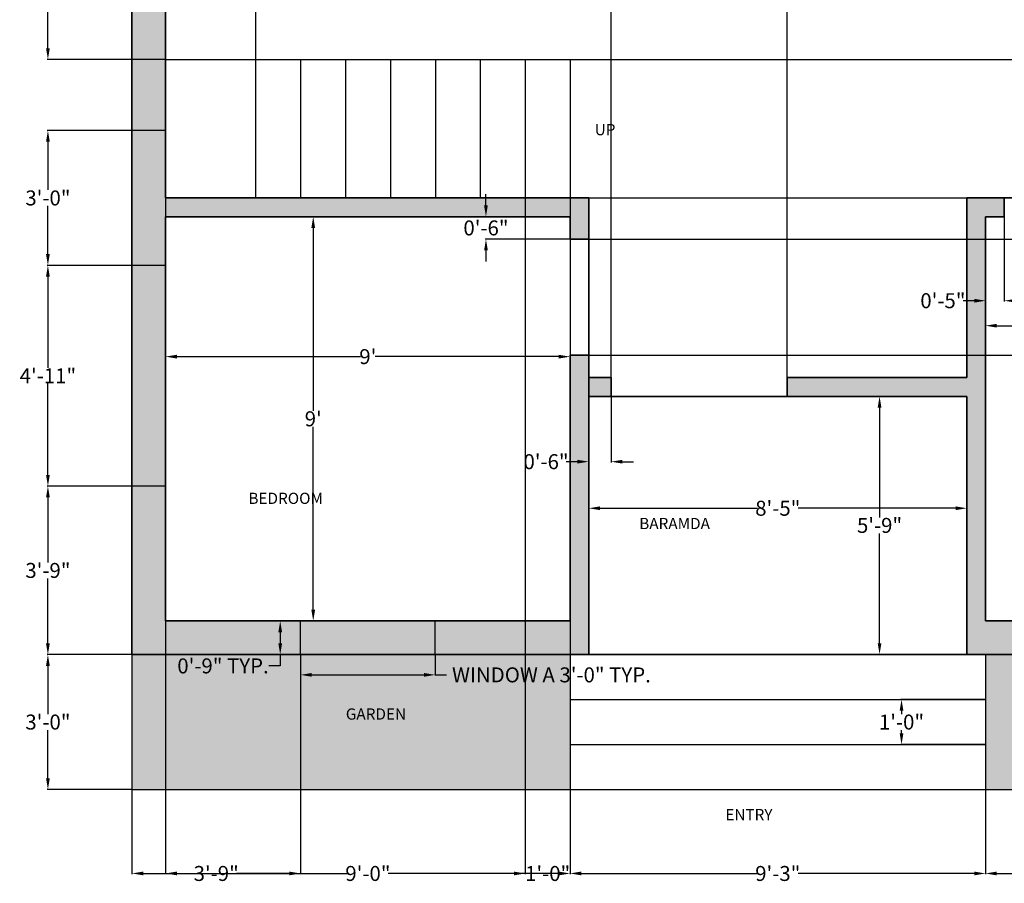
# Model space of a CAD drawing. Units: inches. Extents: x 477 to 929, y 265 to 727.
# Tile 1 of 4: x 477 to 740, y 265 to 496. Entities that reach past the tile are written whole.
import ezdxf

# ---------------------------------------------------------------- set-up
doc = ezdxf.new("R2010")
doc.units = ezdxf.units.IN
doc.header["$MEASUREMENT"] = 0
for name, color, linetype, lineweight, true_color in [('A-ANNO-DIMS', 215, 'Continuous', 18, 0xa953a0), ('A-WALL-PATT', 244, 'Continuous', 13, 0x991b1e), ('L-PLNT-PATT', 114, 'Continuous', 13, 0x139b48)]:
    doc.layers.add(name, color=color, linetype=linetype, lineweight=lineweight, true_color=true_color)
for name, color, linetype, lineweight in [('A-ANNO-TEXT', 3, 'Continuous', 18), ('A-AREA-IDEN', 3, 'Continuous', 25), ('A-FLOR-STRS', 7, 'Continuous', 25), ('A-GLAZ', 4, 'Continuous', 25), ('A-GLAZ-PATT', 7, 'Continuous', 13), ('A-WALL', 7, 'Continuous', 35), ('L-SITE', 7, 'Continuous', 25)]:
    doc.layers.add(name, color=color, linetype=linetype, lineweight=lineweight)
doc.styles.get("Standard").update_dxf_attribs({"font": 'arial.ttf'})
doc.dimstyles.get("Standard").update_dxf_attribs({"dimtxt": 4, "dimasz": 3, "dimexe": 0.18, "dimexo": 0.0625, "dimgap": 0.09, "dimtad": 0, "dimtih": 1, "dimtoh": 1, "dimdec": 0, "dimzin": 0, "dimdsep": 46, "dimlunit": 3, "dimtxsty": 'Standard', "dimcen": 0, "dimadec": 0, "dimazin": 0, "dimtfac": 1, "dimtdec": 0, "dimtofl": 0, "dimtmove": 0, "dimatfit": 3, "dimfxl": 1, "dimtolj": 1, "dimtzin": 0, "dimarcsym": 1})

# ---------------------------------------------------------------- blocks, each defined once
blk = doc.blocks.new('*D1')
at = {"layer": 'A-ANNO-DIMS', "color": 0, "lineweight": -2, "transparency": 16777216}
for p, q in [((553.16, 443.21), (555.92, 443.21)), ((555.74, 440.21), (555.74, 391.34)), ((555.74, 338.21), (555.74, 387.07)), ((555.8, 335.21), (555.92, 335.21))]:
    blk.add_line(p, q, dxfattribs=at)
at = {"layer": 'A-ANNO-DIMS', "color": 0, "transparency": 16777216}
for points in [[(555.24, 440.21), (556.24, 440.21), (555.74, 443.21)], [(555.24, 338.21), (556.24, 338.21), (555.74, 335.21)]]:
    blk.add_solid(points, dxfattribs=at)
at = {"layer": 'Defpoints', "color": 0, "transparency": 16777216}
for p in [(553.09, 443.21), (555.74, 335.21), (555.74, 335.21)]:
    blk.add_point(p, dxfattribs=at)
at = {"layer": 'A-ANNO-DIMS', "color": 0, "transparency": 16777216, "insert": (555.74, 389.21), "char_height": 4, "attachment_point": 5}
blk.add_mtext("\\A1;9'", dxfattribs=at)
blk = doc.blocks.new('*D2')
at = {"layer": 'A-ANNO-DIMS', "color": 0, "lineweight": -2, "transparency": 16777216}
for p, q in [((516.33, 389.27), (516.33, 406)), ((519.33, 405.82), (568.4, 405.82)), ((621.33, 405.82), (572.26, 405.82)), ((624.33, 389.27), (624.33, 406))]:
    blk.add_line(p, q, dxfattribs=at)
at = {"layer": 'A-ANNO-DIMS', "color": 0, "transparency": 16777216}
for points in [[(519.33, 406.32), (519.33, 405.32), (516.33, 405.82)], [(621.33, 406.32), (621.33, 405.32), (624.33, 405.82)]]:
    blk.add_solid(points, dxfattribs=at)
at = {"layer": 'Defpoints', "color": 0, "transparency": 16777216}
for p in [(624.33, 405.82), (516.33, 389.21), (624.33, 389.21)]:
    blk.add_point(p, dxfattribs=at)
at = {"layer": 'A-ANNO-DIMS', "color": 0, "transparency": 16777216, "insert": (570.33, 405.82), "char_height": 4, "attachment_point": 5}
blk.add_mtext("\\A1;9'", dxfattribs=at)
blk = doc.blocks.new('*D3')
at = {"layer": 'A-ANNO-DIMS', "color": 0, "lineweight": -2, "transparency": 16777216}
for p, q in [((629.33, 326.27), (629.33, 365.5)), ((632.33, 365.32), (674.42, 365.32)), ((727.33, 365.32), (685.24, 365.32)), ((730.33, 326.27), (730.33, 365.5))]:
    blk.add_line(p, q, dxfattribs=at)
at = {"layer": 'A-ANNO-DIMS', "color": 0, "transparency": 16777216}
for points in [[(632.33, 365.82), (632.33, 364.82), (629.33, 365.32)], [(727.33, 365.82), (727.33, 364.82), (730.33, 365.32)]]:
    blk.add_solid(points, dxfattribs=at)
at = {"layer": 'Defpoints', "color": 0, "transparency": 16777216}
for p in [(730.33, 365.32), (629.33, 326.21), (730.33, 326.21)]:
    blk.add_point(p, dxfattribs=at)
at = {"layer": 'A-ANNO-DIMS', "color": 0, "transparency": 16777216, "insert": (679.83, 365.32), "char_height": 4, "attachment_point": 5}
blk.add_mtext('\\A1;8\'-5"', dxfattribs=at)
blk = doc.blocks.new('*D4')
at = {"layer": 'A-ANNO-DIMS', "color": 0, "lineweight": -2, "transparency": 16777216}
for p, q in [((730.27, 395.21), (706.83, 395.21)), ((707.01, 392.21), (707.01, 362.87)), ((707.01, 329.27), (707.01, 358.6)), ((730.27, 326.27), (706.83, 326.27))]:
    blk.add_line(p, q, dxfattribs=at)
at = {"layer": 'A-ANNO-DIMS', "color": 0, "transparency": 16777216}
for points in [[(706.51, 392.21), (707.51, 392.21), (707.01, 395.21)], [(706.51, 329.27), (707.51, 329.27), (707.01, 326.27)]]:
    blk.add_solid(points, dxfattribs=at)
at = {"layer": 'Defpoints', "color": 0, "transparency": 16777216}
for p in [(730.33, 395.21), (707.01, 326.27), (730.33, 326.27)]:
    blk.add_point(p, dxfattribs=at)
at = {"layer": 'A-ANNO-DIMS', "color": 0, "transparency": 16777216, "insert": (707.01, 360.74), "char_height": 4, "attachment_point": 5}
blk.add_mtext('\\A1;5\'-9"', dxfattribs=at)
blk = doc.blocks.new('*D5')
at = {"layer": 'A-ANNO-DIMS', "color": 0, "lineweight": -2, "transparency": 16777216}
for p, q in [((735.33, 335.27), (735.33, 414.27)), ((738.33, 414.09), (796.06, 414.09)), ((867.33, 414.09), (809.61, 414.09)), ((870.33, 335.27), (870.33, 414.27))]:
    blk.add_line(p, q, dxfattribs=at)
at = {"layer": 'A-ANNO-DIMS', "color": 0, "transparency": 16777216}
for points in [[(738.33, 414.59), (738.33, 413.59), (735.33, 414.09)], [(867.33, 414.59), (867.33, 413.59), (870.33, 414.09)]]:
    blk.add_solid(points, dxfattribs=at)
at = {"layer": 'Defpoints', "color": 0, "transparency": 16777216}
for p in [(870.33, 414.09), (735.33, 335.21), (870.33, 335.21)]:
    blk.add_point(p, dxfattribs=at)
at = {"layer": 'A-ANNO-DIMS', "color": 0, "transparency": 16777216, "insert": (802.83, 414.09), "char_height": 4, "attachment_point": 5}
blk.add_mtext('\\A1;11\'-3"', dxfattribs=at)
blk = doc.blocks.new('WIN-JAMBS-36IN')
for p, q in [((9, 36), (0, 36)), ((9, 0), (0, 0))]:
    blk.add_line(p, q)
blk = doc.blocks.new('*D23')
at = {"layer": 'A-ANNO-DIMS', "color": 0, "lineweight": -2, "transparency": 16777216}
for p, q in [((552.33, 326.14), (552.33, 320.63)), ((588.33, 326.14), (588.33, 320.63)), ((555.33, 320.81), (585.33, 320.81)), ((588.33, 320.81), (591.33, 320.81))]:
    blk.add_line(p, q, dxfattribs=at)
at = {"layer": 'A-ANNO-DIMS', "color": 0, "transparency": 16777216}
for points in [[(555.33, 321.31), (555.33, 320.31), (552.33, 320.81)], [(585.33, 321.31), (585.33, 320.31), (588.33, 320.81)]]:
    blk.add_solid(points, dxfattribs=at)
at = {"layer": 'Defpoints', "color": 0, "transparency": 16777216}
for p in [(552.33, 326.21), (588.33, 326.21), (588.33, 320.81)]:
    blk.add_point(p, dxfattribs=at)
at = {"layer": 'A-ANNO-DIMS', "color": 0, "transparency": 16777216, "insert": (619.37, 320.81), "char_height": 4, "attachment_point": 5}
blk.add_mtext('\\A1;WINDOW A 3\'-0" TYP.', dxfattribs=at)
blk = doc.blocks.new('*D24')
at = {"layer": 'A-ANNO-DIMS', "color": 0, "lineweight": -2, "transparency": 16777216}
for p, q in [((552.27, 335.21), (546.75, 335.21)), ((546.93, 332.21), (546.93, 329.21)), ((552.27, 326.21), (546.75, 326.21)), ((546.93, 326.21), (546.93, 323.21)), ((546.93, 323.21), (543.93, 323.21))]:
    blk.add_line(p, q, dxfattribs=at)
at = {"layer": 'A-ANNO-DIMS', "color": 0, "transparency": 16777216}
for points in [[(546.43, 332.21), (547.43, 332.21), (546.93, 335.21)], [(546.43, 329.21), (547.43, 329.21), (546.93, 326.21)]]:
    blk.add_solid(points, dxfattribs=at)
at = {"layer": 'Defpoints', "color": 0, "transparency": 16777216}
for p in [(552.33, 335.21), (546.93, 326.21), (552.33, 326.21)]:
    blk.add_point(p, dxfattribs=at)
at = {"layer": 'A-ANNO-DIMS', "color": 0, "transparency": 16777216, "insert": (531.65, 323.21), "char_height": 4, "attachment_point": 5}
blk.add_mtext('\\A1;0\'-9" TYP.', dxfattribs=at)
blk = doc.blocks.new('*D29')
at = {"layer": 'A-ANNO-DIMS', "color": 0, "lineweight": -2, "transparency": 16777216}
for p, q in [((624.43, 485.21), (901.96, 485.21)), ((901.78, 482.21), (901.78, 468.84)), ((901.78, 451.21), (901.78, 464.57)), ((624.43, 448.21), (901.96, 448.21))]:
    blk.add_line(p, q, dxfattribs=at)
at = {"layer": 'A-ANNO-DIMS', "color": 0, "transparency": 16777216}
for points in [[(901.28, 482.21), (902.28, 482.21), (901.78, 485.21)], [(901.28, 451.21), (902.28, 451.21), (901.78, 448.21)]]:
    blk.add_solid(points, dxfattribs=at)
at = {"layer": 'Defpoints', "color": 0, "transparency": 16777216}
for p in [(624.37, 485.21), (901.78, 485.21), (624.37, 448.21)]:
    blk.add_point(p, dxfattribs=at)
at = {"layer": 'A-ANNO-DIMS', "color": 0, "transparency": 16777216, "insert": (901.78, 466.71), "char_height": 4, "attachment_point": 5}
blk.add_mtext('\\A1;3\'-1"', dxfattribs=at)
blk = doc.blocks.new('*D31')
at = {"layer": 'A-ANNO-DIMS', "color": 0, "lineweight": -2, "transparency": 16777216}
for p, q in [((612.368072, 485.142663), (612.368072, 267.575163)), ((624.368072, 485.142663), (624.368072, 267.575163)), ((609.368072, 267.755163), (606.368072, 267.755163)), ((627.368072, 267.755163), (630.368072, 267.755163))]:
    blk.add_line(p, q, dxfattribs=at)
at = {"layer": 'A-ANNO-DIMS', "color": 0, "transparency": 16777216}
for points in [[(609.368072, 268.255163), (609.368072, 267.255163), (612.368072, 267.755163)], [(627.368072, 268.255163), (627.368072, 267.255163), (624.368072, 267.755163)]]:
    blk.add_solid(points, dxfattribs=at)
at = {"layer": 'Defpoints', "color": 0, "transparency": 16777216}
for p in [(612.368072, 485.205163), (624.368072, 485.205163), (624.368072, 267.755163)]:
    blk.add_point(p, dxfattribs=at)
at = {"layer": 'A-ANNO-DIMS', "color": 0, "transparency": 16777216, "insert": (618.368072, 267.755163), "char_height": 4, "attachment_point": 5}
blk.add_mtext('\\A1;1\'-0"', dxfattribs=at)
blk = doc.blocks.new('*D34')
at = {"layer": 'A-ANNO-DIMS', "color": 0, "lineweight": -2, "transparency": 16777216}
for p, q in [((516.33, 448.14), (516.33, 267.58)), ((624.37, 448.14), (624.37, 267.58)), ((519.33, 267.76), (564.94, 267.76)), ((621.37, 267.76), (575.76, 267.76))]:
    blk.add_line(p, q, dxfattribs=at)
at = {"layer": 'A-ANNO-DIMS', "color": 0, "transparency": 16777216}
for points in [[(519.33, 268.26), (519.33, 267.26), (516.33, 267.76)], [(621.37, 268.26), (621.37, 267.26), (624.37, 267.76)]]:
    blk.add_solid(points, dxfattribs=at)
at = {"layer": 'Defpoints', "color": 0, "transparency": 16777216}
for p in [(516.33, 448.21), (624.37, 448.21), (624.37, 267.76)]:
    blk.add_point(p, dxfattribs=at)
at = {"layer": 'A-ANNO-DIMS', "color": 0, "transparency": 16777216, "insert": (570.35, 267.76), "char_height": 4, "attachment_point": 5}
blk.add_mtext('\\A1;9\'-0"', dxfattribs=at)
blk = doc.blocks.new('*D35')
at = {"layer": 'A-ANNO-DIMS', "color": 0, "lineweight": -2, "transparency": 16777216}
for p, q in [((516.27, 521.21), (484.7, 521.21)), ((484.88, 518.21), (484.88, 505.34)), ((484.88, 488.21), (484.88, 501.07)), ((516.27, 485.21), (484.7, 485.21))]:
    blk.add_line(p, q, dxfattribs=at)
at = {"layer": 'A-ANNO-DIMS', "color": 0, "transparency": 16777216}
for points in [[(484.38, 518.21), (485.38, 518.21), (484.88, 521.21)], [(484.38, 488.21), (485.38, 488.21), (484.88, 485.21)]]:
    blk.add_solid(points, dxfattribs=at)
at = {"layer": 'Defpoints', "color": 0, "transparency": 16777216}
for p in [(484.88, 521.21), (516.33, 521.21), (516.33, 485.21)]:
    blk.add_point(p, dxfattribs=at)
at = {"layer": 'A-ANNO-DIMS', "color": 0, "transparency": 16777216, "insert": (484.88, 503.21), "char_height": 4, "attachment_point": 5}
blk.add_mtext('\\A1;3\'-0"', dxfattribs=at)
blk = doc.blocks.new('*D36')
at = {"layer": 'A-ANNO-DIMS', "color": 0, "lineweight": -2, "transparency": 16777216}
for p, q in [((507.27, 326.21), (484.7, 326.21)), ((484.88, 323.21), (484.88, 310.34)), ((484.88, 293.21), (484.88, 306.07)), ((507.27, 290.21), (484.7, 290.21))]:
    blk.add_line(p, q, dxfattribs=at)
at = {"layer": 'A-ANNO-DIMS', "color": 0, "transparency": 16777216}
for points in [[(484.38, 323.21), (485.38, 323.21), (484.88, 326.21)], [(484.38, 293.21), (485.38, 293.21), (484.88, 290.21)]]:
    blk.add_solid(points, dxfattribs=at)
at = {"layer": 'Defpoints', "color": 0, "transparency": 16777216}
for p in [(507.33, 326.21), (484.88, 290.21), (507.33, 290.21)]:
    blk.add_point(p, dxfattribs=at)
at = {"layer": 'A-ANNO-DIMS', "color": 0, "transparency": 16777216, "insert": (484.88, 308.21), "char_height": 4, "attachment_point": 5}
blk.add_mtext('\\A1;3\'-0"', dxfattribs=at)
blk = doc.blocks.new('*D37')
at = {"layer": 'A-ANNO-DIMS', "color": 0, "lineweight": -2, "transparency": 16777216}
for p, q in [((624.33, 290.14), (624.33, 267.58)), ((735.33, 290.14), (735.33, 267.58)), ((627.33, 267.76), (674.43, 267.76)), ((732.33, 267.76), (685.24, 267.76))]:
    blk.add_line(p, q, dxfattribs=at)
at = {"layer": 'A-ANNO-DIMS', "color": 0, "transparency": 16777216}
for points in [[(627.33, 268.26), (627.33, 267.26), (624.33, 267.76)], [(732.33, 268.26), (732.33, 267.26), (735.33, 267.76)]]:
    blk.add_solid(points, dxfattribs=at)
at = {"layer": 'Defpoints', "color": 0, "transparency": 16777216}
for p in [(624.33, 290.21), (735.33, 290.21), (735.33, 267.76)]:
    blk.add_point(p, dxfattribs=at)
at = {"layer": 'A-ANNO-DIMS', "color": 0, "transparency": 16777216, "insert": (679.83, 267.76), "char_height": 4, "attachment_point": 5}
blk.add_mtext('\\A1;9\'-3"', dxfattribs=at)
blk = doc.blocks.new('*D38')
at = {"layer": 'A-ANNO-DIMS', "color": 0, "lineweight": -2, "transparency": 16777216}
for p, q in [((735.27, 314.21), (712.7, 314.21)), ((712.88, 311.21), (712.88, 310.34)), ((712.88, 305.21), (712.88, 306.07)), ((735.27, 302.21), (712.7, 302.21))]:
    blk.add_line(p, q, dxfattribs=at)
at = {"layer": 'A-ANNO-DIMS', "color": 0, "transparency": 16777216}
for points in [[(712.38, 311.21), (713.38, 311.21), (712.88, 314.21)], [(712.38, 305.21), (713.38, 305.21), (712.88, 302.21)]]:
    blk.add_solid(points, dxfattribs=at)
at = {"layer": 'Defpoints', "color": 0, "transparency": 16777216}
for p in [(712.88, 314.21), (735.33, 314.21), (735.33, 302.21)]:
    blk.add_point(p, dxfattribs=at)
at = {"layer": 'A-ANNO-DIMS', "color": 0, "transparency": 16777216, "insert": (712.88, 308.21), "char_height": 4, "attachment_point": 5}
blk.add_mtext('\\A1;1\'-0"', dxfattribs=at)
blk = doc.blocks.new('*D47')
at = {"layer": 'A-ANNO-DIMS', "color": 0, "lineweight": -2, "transparency": 16777216}
for p, q in [((507.27, 371.21), (484.7, 371.21)), ((484.88, 368.21), (484.88, 350.84)), ((484.88, 329.21), (484.88, 346.57)), ((507.27, 326.21), (484.7, 326.21))]:
    blk.add_line(p, q, dxfattribs=at)
at = {"layer": 'A-ANNO-DIMS', "color": 0, "transparency": 16777216}
for points in [[(484.38, 368.21), (485.38, 368.21), (484.88, 371.21)], [(484.38, 329.21), (485.38, 329.21), (484.88, 326.21)]]:
    blk.add_solid(points, dxfattribs=at)
at = {"layer": 'Defpoints', "color": 0, "transparency": 16777216}
for p in [(484.88, 371.21), (507.33, 371.21), (507.33, 326.21)]:
    blk.add_point(p, dxfattribs=at)
at = {"layer": 'A-ANNO-DIMS', "color": 0, "transparency": 16777216, "insert": (484.88, 348.71), "char_height": 4, "attachment_point": 5}
blk.add_mtext('\\A1;3\'-9"', dxfattribs=at)
blk = doc.blocks.new('*D48')
at = {"layer": 'A-ANNO-DIMS', "color": 0, "lineweight": -2, "transparency": 16777216}
for p, q in [((507.27, 466.21), (484.7, 466.21)), ((484.88, 463.21), (484.88, 450.34)), ((484.88, 433.21), (484.88, 446.07)), ((507.27, 430.21), (484.7, 430.21))]:
    blk.add_line(p, q, dxfattribs=at)
at = {"layer": 'A-ANNO-DIMS', "color": 0, "transparency": 16777216}
for points in [[(484.38, 463.21), (485.38, 463.21), (484.88, 466.21)], [(484.38, 433.21), (485.38, 433.21), (484.88, 430.21)]]:
    blk.add_solid(points, dxfattribs=at)
at = {"layer": 'Defpoints', "color": 0, "transparency": 16777216}
for p in [(484.88, 466.21), (507.33, 466.21), (507.33, 430.21)]:
    blk.add_point(p, dxfattribs=at)
at = {"layer": 'A-ANNO-DIMS', "color": 0, "transparency": 16777216, "insert": (484.88, 448.21), "char_height": 4, "attachment_point": 5}
blk.add_mtext('\\A1;3\'-0"', dxfattribs=at)
blk = doc.blocks.new('*D49')
at = {"layer": 'A-ANNO-DIMS', "color": 0, "lineweight": -2, "transparency": 16777216}
for p, q in [((507.27, 430.21), (484.7, 430.21)), ((484.88, 427.21), (484.88, 402.8)), ((484.88, 374.21), (484.88, 398.61)), ((507.27, 371.21), (484.7, 371.21))]:
    blk.add_line(p, q, dxfattribs=at)
at = {"layer": 'A-ANNO-DIMS', "color": 0, "transparency": 16777216}
for points in [[(484.38, 427.21), (485.38, 427.21), (484.88, 430.21)], [(484.38, 374.21), (485.38, 374.21), (484.88, 371.21)]]:
    blk.add_solid(points, dxfattribs=at)
at = {"layer": 'Defpoints', "color": 0, "transparency": 16777216}
for p in [(484.88, 430.21), (507.33, 430.21), (507.33, 371.21)]:
    blk.add_point(p, dxfattribs=at)
at = {"layer": 'A-ANNO-DIMS', "color": 0, "transparency": 16777216, "insert": (484.88, 400.71), "char_height": 4, "attachment_point": 5}
blk.add_mtext('\\A1;4\'-11"', dxfattribs=at)
blk = doc.blocks.new('*D54')
at = {"layer": 'A-ANNO-DIMS', "color": 0, "lineweight": -2, "transparency": 16777216}
for p, q in [((507.33, 326.14), (507.33, 267.58)), ((552.33, 326.14), (552.33, 267.58)), ((510.33, 267.76), (524.43, 267.76)), ((549.33, 267.76), (535.24, 267.76))]:
    blk.add_line(p, q, dxfattribs=at)
at = {"layer": 'A-ANNO-DIMS', "color": 0, "transparency": 16777216}
for points in [[(510.33, 268.26), (510.33, 267.26), (507.33, 267.76)], [(549.33, 268.26), (549.33, 267.26), (552.33, 267.76)]]:
    blk.add_solid(points, dxfattribs=at)
at = {"layer": 'Defpoints', "color": 0, "transparency": 16777216}
for p in [(507.33, 326.21), (552.33, 326.21), (552.33, 267.76)]:
    blk.add_point(p, dxfattribs=at)
at = {"layer": 'A-ANNO-DIMS', "color": 0, "transparency": 16777216, "insert": (529.83, 267.76), "char_height": 4, "attachment_point": 5}
blk.add_mtext('\\A1;3\'-9"', dxfattribs=at)
blk = doc.blocks.new('*D55')
at = {"layer": 'A-ANNO-DIMS', "color": 0, "lineweight": -2, "transparency": 16777216}
for p, q in [((735.33, 326.14), (735.33, 267.58)), ((766.33, 326.14), (766.33, 267.58)), ((738.33, 267.76), (745.39, 267.76)), ((763.33, 267.76), (756.27, 267.76))]:
    blk.add_line(p, q, dxfattribs=at)
at = {"layer": 'A-ANNO-DIMS', "color": 0, "transparency": 16777216}
for points in [[(738.33, 268.26), (738.33, 267.26), (735.33, 267.76)], [(763.33, 268.26), (763.33, 267.26), (766.33, 267.76)]]:
    blk.add_solid(points, dxfattribs=at)
at = {"layer": 'Defpoints', "color": 0, "transparency": 16777216}
for p in [(735.33, 326.21), (766.33, 326.21), (766.33, 267.76)]:
    blk.add_point(p, dxfattribs=at)
at = {"layer": 'A-ANNO-DIMS', "color": 0, "transparency": 16777216, "insert": (750.83, 267.76), "char_height": 4, "attachment_point": 5}
blk.add_mtext('\\A1;2\'-7"', dxfattribs=at)
blk = doc.blocks.new('*D57')
at = {"layer": 'A-ANNO-DIMS', "color": 0, "lineweight": -2, "transparency": 16777216}
for p, q in [((635.33, 400.27), (635.33, 720.84)), ((638.33, 720.66), (651.87, 720.66)), ((679.33, 720.66), (665.79, 720.66)), ((682.33, 400.27), (682.33, 720.84))]:
    blk.add_line(p, q, dxfattribs=at)
at = {"layer": 'A-ANNO-DIMS', "color": 0, "transparency": 16777216}
for points in [[(638.33, 721.16), (638.33, 720.16), (635.33, 720.66)], [(679.33, 721.16), (679.33, 720.16), (682.33, 720.66)]]:
    blk.add_solid(points, dxfattribs=at)
at = {"layer": 'Defpoints', "color": 0, "transparency": 16777216}
for p in [(682.33, 720.66), (635.33, 400.21), (682.33, 400.21)]:
    blk.add_point(p, dxfattribs=at)
at = {"layer": 'A-ANNO-DIMS', "color": 0, "transparency": 16777216, "insert": (658.83, 720.66), "char_height": 4, "attachment_point": 5}
blk.add_mtext('\\A1;3\'-11"', dxfattribs=at)
blk = doc.blocks.new('*D58')
at = {"layer": 'A-ANNO-DIMS', "color": 0, "lineweight": -2, "transparency": 16777216}
for p, q in [((629.4, 437.21), (901.96, 437.21)), ((901.78, 434.21), (901.78, 423.8)), ((901.78, 409.21), (901.78, 419.61)), ((629.4, 406.21), (901.96, 406.21))]:
    blk.add_line(p, q, dxfattribs=at)
at = {"layer": 'A-ANNO-DIMS', "color": 0, "transparency": 16777216}
for points in [[(901.28, 434.21), (902.28, 434.21), (901.78, 437.21)], [(901.28, 409.21), (902.28, 409.21), (901.78, 406.21)]]:
    blk.add_solid(points, dxfattribs=at)
at = {"layer": 'Defpoints', "color": 0, "transparency": 16777216}
for p in [(629.33, 437.21), (901.78, 437.21), (629.33, 406.21)]:
    blk.add_point(p, dxfattribs=at)
at = {"layer": 'A-ANNO-DIMS', "color": 0, "transparency": 16777216, "insert": (901.78, 421.71), "char_height": 4, "attachment_point": 5}
blk.add_mtext('\\A1;2\'-7"', dxfattribs=at)
blk = doc.blocks.new('*D64')
at = {"layer": 'A-ANNO-DIMS', "color": 0, "lineweight": -2, "transparency": 16777216}
for p, q in [((629.33, 400.14), (629.33, 377.58)), ((635.33, 400.14), (635.33, 377.58)), ((626.33, 377.76), (623.33, 377.76)), ((638.33, 377.76), (641.33, 377.76))]:
    blk.add_line(p, q, dxfattribs=at)
at = {"layer": 'A-ANNO-DIMS', "color": 0, "transparency": 16777216}
for points in [[(626.33, 378.26), (626.33, 377.26), (629.33, 377.76)], [(638.33, 378.26), (638.33, 377.26), (635.33, 377.76)]]:
    blk.add_solid(points, dxfattribs=at)
at = {"layer": 'Defpoints', "color": 0, "transparency": 16777216}
for p in [(629.33, 400.21), (635.33, 400.21), (629.33, 377.76)]:
    blk.add_point(p, dxfattribs=at)
at = {"layer": 'A-ANNO-DIMS', "color": 0, "transparency": 16777216, "insert": (617.93, 377.76), "char_height": 4, "attachment_point": 5}
blk.add_mtext('\\A1;0\'-6"', dxfattribs=at)
blk = doc.blocks.new('*D65')
at = {"layer": 'A-ANNO-DIMS', "color": 0, "lineweight": -2, "transparency": 16777216}
for p, q in [((735.33, 443.14), (735.33, 420.58)), ((740.33, 443.14), (740.33, 420.58)), ((732.33, 420.76), (729.33, 420.76)), ((743.33, 420.76), (746.33, 420.76))]:
    blk.add_line(p, q, dxfattribs=at)
at = {"layer": 'A-ANNO-DIMS', "color": 0, "transparency": 16777216}
for points in [[(732.33, 421.26), (732.33, 420.26), (735.33, 420.76)], [(743.33, 421.26), (743.33, 420.26), (740.33, 420.76)]]:
    blk.add_solid(points, dxfattribs=at)
at = {"layer": 'Defpoints', "color": 0, "transparency": 16777216}
for p in [(735.33, 443.21), (740.33, 443.21), (735.33, 420.76)]:
    blk.add_point(p, dxfattribs=at)
at = {"layer": 'A-ANNO-DIMS', "color": 0, "transparency": 16777216, "insert": (723.93, 420.76), "char_height": 4, "attachment_point": 5}
blk.add_mtext('\\A1;0\'-5"', dxfattribs=at)
blk = doc.blocks.new('*D67')
at = {"layer": 'A-ANNO-DIMS', "color": 0, "lineweight": -2, "transparency": 16777216}
for p, q in [((601.883739, 446.205163), (601.883739, 449.205163)), ((624.271239, 443.205163), (601.703739, 443.205163)), ((624.271239, 437.205163), (601.703739, 437.205163)), ((601.883739, 434.205163), (601.883739, 431.205163))]:
    blk.add_line(p, q, dxfattribs=at)
at = {"layer": 'A-ANNO-DIMS', "color": 0, "transparency": 16777216}
for points in [[(601.383739, 446.205163), (602.383739, 446.205163), (601.883739, 443.205163)], [(601.383739, 434.205163), (602.383739, 434.205163), (601.883739, 437.205163)]]:
    blk.add_solid(points, dxfattribs=at)
at = {"layer": 'Defpoints', "color": 0, "transparency": 16777216}
for p in [(601.883739, 443.205163), (624.333739, 443.205163), (624.333739, 437.205163)]:
    blk.add_point(p, dxfattribs=at)
at = {"layer": 'A-ANNO-DIMS', "color": 0, "transparency": 16777216, "insert": (601.883739, 440.205163), "char_height": 4, "attachment_point": 5}
blk.add_mtext('\\A1;0\'-6"', dxfattribs=at)

msp = doc.modelspace()

# ---------------------------------------------------------------- hatches: boundary and pattern name
at = {"layer": 'A-GLAZ-PATT'}
h = msp.add_hatch(color=256, dxfattribs=at)
h.dxf.hatch_style = 1
h.paths.add_polyline_path([(588.33, 698.21), (552.33, 698.21), (552.33, 689.21), (588.33, 689.21)])
h.paths.add_polyline_path([(659.33, 698.21), (647.33, 698.21), (647.33, 689.21), (659.33, 689.21)])
h.paths.add_polyline_path([(712.33, 698.21), (700.33, 698.21), (700.33, 689.21), (712.33, 689.21)])
h.paths.add_polyline_path([(834.33, 698.21), (771.33, 698.21), (771.33, 689.21), (834.33, 689.21)])
h.paths.add_polyline_path([(879.33, 653.21), (870.33, 653.21), (870.33, 598.21), (879.33, 598.21)])
h.paths.add_polyline_path([(879.33, 521.21), (870.33, 521.21), (870.33, 484.21), (879.33, 484.21)])
h.paths.add_polyline_path([(879.33, 407.21), (870.33, 407.21), (870.33, 371.21), (879.33, 371.21)])
h.paths.add_polyline_path([(834.33, 335.21), (766.33, 335.21), (766.33, 326.21), (834.33, 326.21)])
h.paths.add_polyline_path([(588.33, 335.21), (552.33, 335.21), (552.33, 326.21), (588.33, 326.21)])
h.paths.add_polyline_path([(516.33, 430.21), (507.33, 430.21), (507.33, 371.21), (516.33, 371.21)])
h.paths.add_polyline_path([(516.33, 539.21), (507.33, 539.21), (507.33, 466.21), (516.33, 466.21)])
h.paths.add_polyline_path([(516.33, 653.21), (507.33, 653.21), (507.33, 598.21), (516.33, 598.21)])
at = {"layer": 'A-WALL-PATT'}
h = msp.add_hatch(color=256, dxfattribs=at)
h.dxf.hatch_style = 1
h.paths.add_polyline_path([(516.33, 598.21), (507.33, 598.21), (507.33, 539.21), (516.33, 539.21), (516.33, 557.21), (570.33, 557.21), (570.33, 562.21), (516.33, 562.21)])
h.paths.add_polyline_path([(552.33, 698.21), (507.33, 698.21), (507.33, 653.21), (516.33, 653.21), (516.33, 689.21), (552.33, 689.21)])
h.paths.add_polyline_path([(647.33, 698.21), (588.33, 698.21), (588.33, 689.21), (647.33, 689.21)])
h.paths.add_polyline_path([(700.33, 698.21), (659.33, 698.21), (659.33, 689.21), (700.33, 689.21)])
h.paths.add_polyline_path([(771.33, 698.21), (712.33, 698.21), (712.33, 689.21), (771.33, 689.21)])
h.paths.add_polyline_path([(879.33, 698.21), (834.33, 698.21), (834.33, 689.21), (870.33, 689.21), (870.33, 653.21), (879.33, 653.21)])
h.paths.add_polyline_path([(879.33, 598.21), (870.33, 598.21), (870.33, 562.21), (735.33, 562.21), (735.33, 568.21), (730.33, 568.21), (730.33, 557.21), (793.33, 557.21), (793.33, 551.21), (798.33, 551.21), (798.33, 557.21), (870.33, 557.21), (870.33, 521.21), (879.33, 521.21)])
h.paths.add_polyline_path([(879.33, 484.21), (870.33, 484.21), (870.33, 448.21), (798.33, 448.21), (798.33, 495.83), (793.33, 495.83), (793.33, 448.21), (788.33, 448.21), (788.33, 443.21), (870.33, 443.21), (870.33, 407.21), (879.33, 407.21)])
h.paths.add_polyline_path([(735.33, 443.21), (740.33, 443.21), (740.33, 448.21), (730.33, 448.21), (730.33, 400.21), (682.33, 400.21), (682.33, 395.21), (730.33, 395.21), (730.33, 326.21), (766.33, 326.21), (766.33, 335.21), (735.33, 335.21)])
h.paths.add_polyline_path([(879.33, 371.21), (870.33, 371.21), (870.33, 335.21), (834.33, 335.21), (834.33, 326.21), (879.33, 326.21)])
h.paths.add_polyline_path([(516.33, 466.21), (507.33, 466.21), (507.33, 430.21), (516.33, 430.21), (516.33, 443.21), (624.33, 443.21), (624.33, 437.21), (629.33, 437.21), (629.33, 448.21), (516.33, 448.21)])
h.paths.add_polyline_path([(629.33, 600.21), (700.33, 600.21), (700.33, 605.21), (682.33, 605.21), (682.33, 689.21), (677.33, 689.21), (677.33, 605.21), (629.33, 605.21), (629.33, 611.21), (624.33, 611.21), (624.33, 562.21), (618.33, 562.21), (618.33, 557.21), (629.33, 557.21)])
h.paths.add_polyline_path([(629.33, 689.21), (624.33, 689.21), (624.33, 653.21), (629.33, 653.21)], flags=17)
h = msp.add_hatch(color=256, dxfattribs=at)
h.dxf.hatch_style = 1
h.paths.add_polyline_path([(516.33, 371.21), (507.33, 371.21), (507.33, 326.21), (552.33, 326.21), (552.33, 335.21), (516.33, 335.21)])
h.paths.add_polyline_path([(629.33, 395.21), (635.33, 395.21), (635.33, 400.21), (629.33, 400.21), (629.33, 406.21), (624.33, 406.21), (624.33, 335.21), (588.33, 335.21), (588.33, 326.21), (629.33, 326.21)])
at = {"layer": 'L-PLNT-PATT'}
h = msp.add_hatch(dxfattribs=at)
h.set_pattern_fill('GRASS', color=256, scale=5)
h.paths.add_polyline_path([(624.33, 326.21), (507.33, 326.21), (507.33, 290.21), (624.33, 290.21)])
h.paths.add_polyline_path([(879.33, 326.21), (735.33, 326.21), (735.33, 290.21), (879.33, 290.21)])
h.paths.add_polyline_path([(790.59, 308.02), (810.07, 308.02), (810.07, 312.68), (790.59, 312.68)], flags=24)

# ---------------------------------------------------------------- linework, layer by layer
at = {"layer": 'A-FLOR-STRS'}
for p, q in [((540.37, 557.21), (540.37, 448.21)), ((516.33, 485.21), (624.37, 485.21)), ((552.37, 485.21), (552.37, 448.21)), ((564.37, 485.21), (564.37, 448.21)), ((576.37, 485.21), (576.37, 448.21)), ((588.37, 485.21), (588.37, 448.21)), ((600.37, 485.21), (600.37, 448.21)), ((612.37, 485.21), (612.37, 448.21)), ((624.37, 485.21), (624.37, 448.21)), ((624.33, 314.21), (735.33, 314.21)), ((624.33, 302.21), (735.33, 302.21))]:
    msp.add_line(p, q, dxfattribs=at)
at = {"layer": 'A-GLAZ'}
for p, q in [((516.33, 466.21), (507.33, 466.21)), ((516.33, 430.21), (507.33, 430.21)), ((516.33, 371.21), (507.33, 371.21))]:
    msp.add_line(p, q, dxfattribs=at)
at = {"layer": 'A-WALL'}
for p, q in [((507.33, 326.21), (507.33, 698.21)), ((507.33, 698.21), (507.33, 326.21)), ((516.33, 448.21), (516.33, 557.21)), ((629.33, 448.21), (516.33, 448.21)), ((629.33, 400.21), (629.33, 448.21)), ((730.33, 400.21), (730.33, 448.21)), ((793.33, 448.21), (730.33, 448.21)), ((740.33, 443.21), (740.33, 448.21)), ((516.33, 335.21), (516.33, 443.21)), ((624.33, 443.21), (516.33, 443.21)), ((624.33, 437.21), (624.33, 443.21)), ((624.33, 437.21), (624.33, 443.21)), ((735.33, 335.21), (735.33, 443.21)), ((740.33, 443.21), (735.33, 443.21)), ((629.33, 437.21), (624.33, 437.21)), ((516.33, 430.21), (516.33, 389.27)), ((735.33, 335.21), (735.33, 414.09)), ((624.33, 335.21), (624.33, 406.21)), ((624.33, 335.21), (624.33, 406.21)), ((629.33, 406.21), (624.33, 406.21)), ((624.33, 389.21), (624.33, 406.21)), ((629.33, 326.21), (629.33, 406.21)), ((635.33, 400.21), (629.33, 400.21)), ((635.33, 395.21), (635.33, 400.21)), ((730.33, 400.21), (682.33, 400.21)), ((682.33, 395.21), (682.33, 400.21)), ((730.33, 395.21), (629.33, 395.21)), ((706.83, 395.21), (730.33, 395.21)), ((730.33, 326.21), (730.33, 395.21)), ((629.33, 365.32), (629.33, 326.27)), ((730.33, 365.5), (730.33, 326.21)), ((624.33, 335.21), (516.33, 335.21)), ((870.33, 335.21), (735.33, 335.21)), ((507.33, 326.21), (879.33, 326.21))]:
    msp.add_line(p, q, dxfattribs=at)
at = {"layer": 'L-SITE'}
for p, q in [((507.33, 326.21), (507.33, 290.21)), ((624.33, 326.21), (624.33, 290.21)), ((735.33, 326.21), (735.33, 290.21)), ((507.33, 290.21), (879.33, 290.21))]:
    msp.add_line(p, q, dxfattribs=at)

# ---------------------------------------------------------------- block references
at = {"layer": 'A-GLAZ', "rotation": 270.0000000000003}
msp.add_blockref('WIN-JAMBS-36IN', (552.33, 335.21), dxfattribs=at)

# ---------------------------------------------------------------- texts
at = {"layer": 'A-ANNO-TEXT'}
for s, p in [('UP', (630.93, 464.96)), ('ENTRY', (665.82, 281.98))]:
    msp.add_text(s, height=3, dxfattribs=at).set_placement(p)
at = {"layer": 'A-AREA-IDEN'}
for s, p in [('BARAMDA', (642.82, 359.74)), ('GARDEN', (564.45, 308.85))]:
    msp.add_text(s, height=3, dxfattribs=at).set_placement(p)
at = {"layer": 'A-AREA-IDEN', "insert": (538.43, 369.47), "char_height": 3, "attachment_point": 1}
msp.add_mtext_dynamic_manual_height_columns('BEDROOM', width=70.7384, gutter_width=1, heights=[0], dxfattribs=at)

# ---------------------------------------------------------------- dimensions: what is measured, and where the dimension line sits
at = {"layer": 'A-ANNO-DIMS'}
for base, p1, p2, override, picture, middle in [((682.33, 720.66), (635.33, 400.21), (682.33, 400.21), {"dimdec": 1, "dimlfac": 1, "dimrnd": 0, "dimzin": 1, "dimdsep": 46, "dimlunit": 4, "dimfrac": 2}, '*D57', (658.83, 720.66)), ((624.37, 267.76), (612.37, 485.21), (624.37, 485.21), {"dimdec": 1, "dimlfac": 1, "dimrnd": 0, "dimzin": 1, "dimdsep": 46, "dimlunit": 4, "dimfrac": 2}, '*D31', (618.37, 267.76)), ((624.37, 267.76), (516.33, 448.21), (624.37, 448.21), {"dimdec": 1, "dimlfac": 1, "dimrnd": 0, "dimzin": 1, "dimdsep": 46, "dimlunit": 4, "dimfrac": 2}, '*D34', (570.35, 267.76)), ((870.33, 414.09), (735.33, 335.21), (870.33, 335.21), {"dimclrd": 0, "dimclre": 0, "dimclrt": 0}, '*D5', (802.83, 414.09)), ((624.33, 405.82), (516.33, 389.21), (624.33, 389.21), {"dimclrd": 0, "dimclre": 0, "dimclrt": 0}, '*D2', (570.33, 405.82)), ((730.33, 365.32), (629.33, 326.21), (730.33, 326.21), {"dimclrd": 0, "dimclre": 0, "dimclrt": 0}, '*D3', (679.83, 365.32)), ((552.33, 267.76), (507.33, 326.21), (552.33, 326.21), {"dimdec": 1, "dimlfac": 1, "dimrnd": 0, "dimzin": 1, "dimdsep": 46, "dimlunit": 4, "dimfrac": 2}, '*D54', (529.83, 267.76)), ((766.33, 267.76), (735.33, 326.21), (766.33, 326.21), {"dimdec": 1, "dimlfac": 1, "dimrnd": 0, "dimzin": 1, "dimdsep": 46, "dimlunit": 4, "dimfrac": 2}, '*D55', (750.83, 267.76)), ((735.33, 267.76), (624.33, 290.21), (735.33, 290.21), {"dimdec": 1, "dimlfac": 1, "dimrnd": 0, "dimzin": 1, "dimdsep": 46, "dimlunit": 4, "dimfrac": 2}, '*D37', (679.83, 267.76))]:
    dim = msp.add_linear_dim(base=base, p1=p1, p2=p2, dimstyle='Standard', override=override, dxfattribs=at)
    dim.commit()
    dim.dimension.update_dxf_attribs({"geometry": picture, "text_midpoint": middle})
for base, p1, p2, angle, override, picture, middle in [((484.88, 521.21), (516.33, 485.21), (516.33, 521.21), 90, {"dimdec": 1, "dimlfac": 1, "dimrnd": 0, "dimzin": 1, "dimdsep": 46, "dimlunit": 4, "dimfrac": 2}, '*D35', (484.88, 503.21)), ((901.78, 485.21), (624.37, 448.21), (624.37, 485.21), 90, {"dimdec": 1, "dimlfac": 1, "dimrnd": 0, "dimzin": 1, "dimdsep": 46, "dimlunit": 4, "dimfrac": 2}, '*D29', (901.78, 466.71)), ((484.88, 466.21), (507.33, 430.21), (507.33, 466.21), 90, {"dimdec": 1, "dimlfac": 1, "dimrnd": 0, "dimzin": 1, "dimdsep": 46, "dimlunit": 4, "dimfrac": 2}, '*D48', (484.88, 448.21)), ((601.88, 443.21), (624.33, 437.21), (624.33, 443.21), 90, {"dimdec": 1, "dimlfac": 1, "dimrnd": 0, "dimzin": 1, "dimdsep": 46, "dimlunit": 4, "dimfrac": 2}, '*D67', (601.88, 440.21)), ((555.74, 335.21), (553.09, 443.21), (555.74, 335.21), 90, {"dimclrd": 0, "dimclre": 0, "dimclrt": 0}, '*D1', (555.74, 389.21)), ((735.33, 420.76), (740.33, 443.21), (735.33, 443.21), 180, {"dimdec": 1, "dimlfac": 1, "dimrnd": 0, "dimzin": 1, "dimdsep": 46, "dimlunit": 4, "dimfrac": 2}, '*D65', (723.93, 420.76)), ((901.78, 437.21), (629.33, 406.21), (629.33, 437.21), 90, {"dimdec": 1, "dimlfac": 1, "dimrnd": 0, "dimzin": 1, "dimdsep": 46, "dimlunit": 4, "dimfrac": 2}, '*D58', (901.78, 421.71)), ((484.88, 430.21), (507.33, 371.21), (507.33, 430.21), 90, {"dimdec": 1, "dimlfac": 1, "dimrnd": 0, "dimzin": 1, "dimdsep": 46, "dimlunit": 4, "dimfrac": 2}, '*D49', (484.88, 400.71)), ((629.33, 377.76), (635.33, 400.21), (629.33, 400.21), 180, {"dimdec": 1, "dimlfac": 1, "dimrnd": 0, "dimzin": 1, "dimdsep": 46, "dimlunit": 4, "dimfrac": 2}, '*D64', (617.93, 377.76)), ((707.01, 326.27), (730.33, 395.21), (730.33, 326.27), 90, {"dimclrd": 0, "dimclre": 0, "dimclrt": 0}, '*D4', (707.01, 360.74)), ((484.88, 371.21), (507.33, 326.21), (507.33, 371.21), 90, {"dimdec": 1, "dimlfac": 1, "dimrnd": 0, "dimzin": 1, "dimdsep": 46, "dimlunit": 4, "dimfrac": 2}, '*D47', (484.88, 348.71)), ((484.88, 290.21), (507.33, 326.21), (507.33, 290.21), 90, {"dimdec": 1, "dimlfac": 1, "dimrnd": 0, "dimzin": 1, "dimdsep": 46, "dimlunit": 4, "dimfrac": 2}, '*D36', (484.88, 308.21)), ((712.88, 314.21), (735.33, 302.21), (735.33, 314.21), 90, {"dimdec": 1, "dimlfac": 1, "dimrnd": 0, "dimzin": 1, "dimdsep": 46, "dimlunit": 4, "dimfrac": 2}, '*D38', (712.88, 308.21))]:
    dim = msp.add_linear_dim(base=base, p1=p1, p2=p2, angle=angle, dimstyle='Standard', override=override, dxfattribs=at)
    dim.commit()
    dim.dimension.update_dxf_attribs({"geometry": picture, "text_midpoint": middle})
for base, p1, p2, angle, text, picture, middle in [((546.93, 326.21), (552.33, 335.21), (552.33, 326.21), 270, '<> TYP.', '*D24', (531.65, 323.21)), ((588.33, 320.81), (552.33, 326.21), (588.33, 326.21), 0, 'WINDOW A <> TYP.', '*D23', (619.37, 320.81))]:
    dim = msp.add_linear_dim(base=base, p1=p1, p2=p2, angle=angle, text=text, dimstyle='Standard', override={"dimdec": 1, "dimlfac": 1, "dimrnd": 0, "dimzin": 1, "dimdsep": 46, "dimlunit": 4, "dimfrac": 2}, dxfattribs=at)
    dim.commit()
    dim.dimension.update_dxf_attribs({"geometry": picture, "text_midpoint": middle})

doc.saveas('drawing.dxf')
